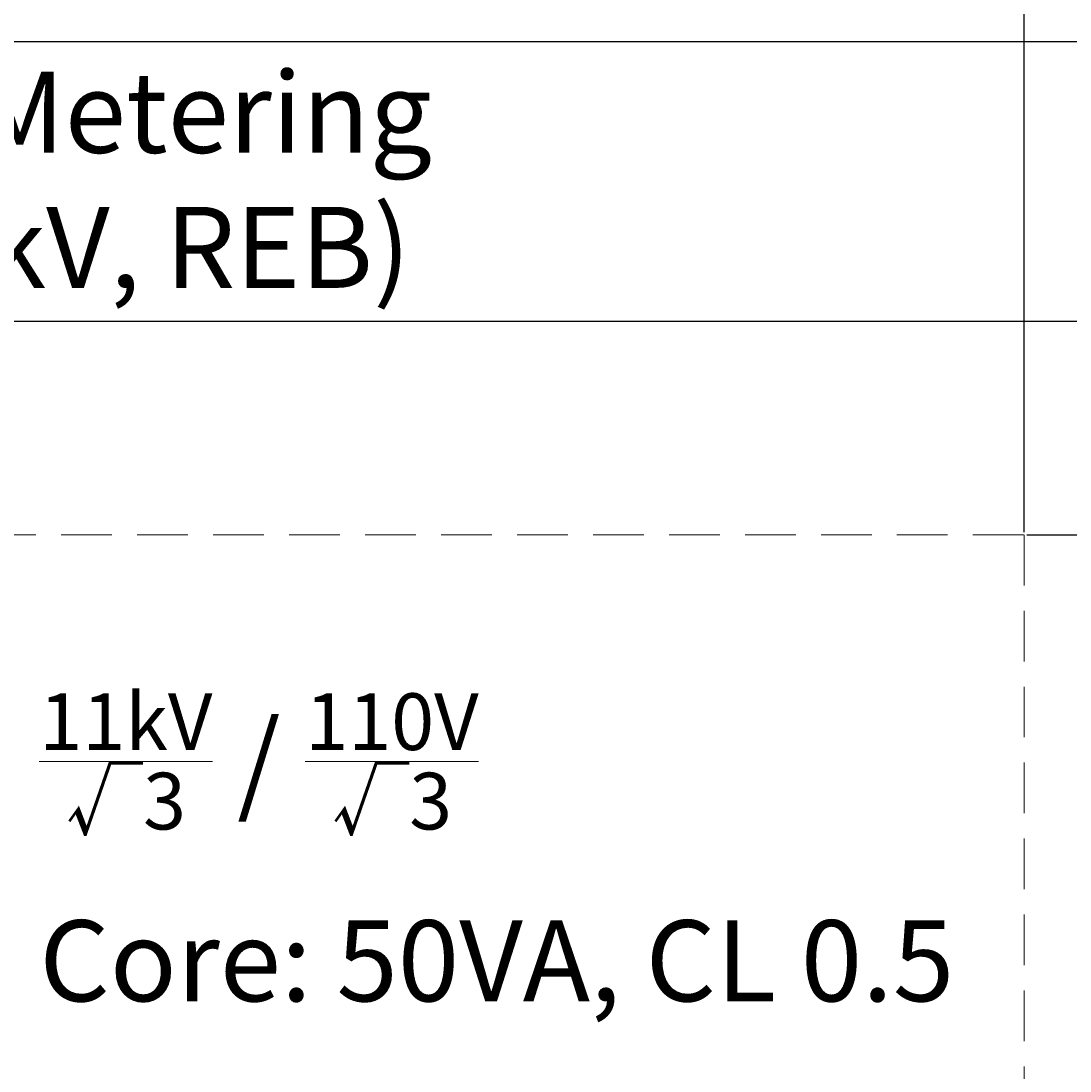
# Model space of a CAD drawing. Units: inches. Extents: x 412 to 584, y 208 to 437.
# Tile 26 of 28: x 514 to 540, y 387 to 413. Entities that reach past the tile are written whole.
import ezdxf

# ---------------------------------------------------------------- set-up
doc = ezdxf.new("R2010")
doc.units = ezdxf.units.IN
doc.header["$MEASUREMENT"] = 0
doc.linetypes.add('HIDDEN', pattern=[0.375, 0.25, -0.125])
for name, color, linetype, lineweight in [('A-ANNO-DIMS', 2, 'Continuous', 18), ('E-ANNO-TEXT', 7, 'Continuous', 18), ('E-ENCL-HIDN', 3, 'HIDDEN', 18)]:
    doc.layers.add(name, color=color, linetype=linetype, lineweight=lineweight)
doc.styles.get("Standard").update_dxf_attribs({"font": 'arial.ttf'})
doc.dimstyles.get("Standard").update_dxf_attribs({"dimtxt": 0.18, "dimasz": 0.18, "dimexe": 0.18, "dimexo": 0.0625, "dimgap": 0.09, "dimtad": 0, "dimtih": 1, "dimtoh": 1, "dimdec": 4, "dimzin": 0, "dimdsep": 46, "dimtxsty": 'Standard', "dimcen": 0.09, "dimadec": 0, "dimazin": 0, "dimtfac": 1, "dimtdec": 4, "dimtofl": 0, "dimtmove": 0, "dimatfit": 3, "dimfxl": 1, "dimtolj": 1, "dimtzin": 0, "dimarcsym": 0})

# ---------------------------------------------------------------- blocks, each defined once
blk = doc.blocks.new('*D17')
at = {"layer": 'A-ANNO-DIMS', "color": 0, "lineweight": -2, "transparency": 16777216}
for p, q in [((497.715, 426.185), (583.674, 426.185)), ((583.494, 426.005), (583.494, 323.031)), ((583.494, 219.693), (583.494, 322.667)), ((550.198, 219.513), (583.674, 219.513))]:
    blk.add_line(p, q, dxfattribs=at)
at = {"layer": 'A-ANNO-DIMS', "color": 0, "transparency": 16777216}
for points in [[(583.464, 426.005), (583.524, 426.005), (583.494, 426.185)], [(583.464, 219.693), (583.524, 219.693), (583.494, 219.513)]]:
    blk.add_solid(points, dxfattribs=at)
at = {"layer": 'Defpoints', "color": 0, "transparency": 16777216}
for p in [(497.652, 426.185), (550.135, 219.513), (583.494, 219.513)]:
    blk.add_point(p, dxfattribs=at)
at = {"layer": 'A-ANNO-DIMS', "color": 0, "transparency": 16777216, "insert": (583.494, 322.849), "char_height": 0.18, "attachment_point": 5}
blk.add_mtext('\\A1;206.67', dxfattribs=at)
blk = doc.blocks.new('*D20')
at = {"layer": 'A-ANNO-DIMS', "color": 0, "lineweight": -2, "transparency": 16777216}
for p, q in [((507.316, 412.35), (583.674, 412.35)), ((583.494, 412.17), (583.494, 406.444)), ((583.494, 400.355), (583.494, 406.08)), ((538.681, 400.175), (583.674, 400.175))]:
    blk.add_line(p, q, dxfattribs=at)
at = {"layer": 'A-ANNO-DIMS', "color": 0, "transparency": 16777216}
for points in [[(583.464, 412.17), (583.524, 412.17), (583.494, 412.35)], [(583.464, 400.355), (583.524, 400.355), (583.494, 400.175)]]:
    blk.add_solid(points, dxfattribs=at)
at = {"layer": 'Defpoints', "color": 0, "transparency": 16777216}
for p in [(507.254, 412.35), (538.619, 400.175), (583.494, 400.175)]:
    blk.add_point(p, dxfattribs=at)
at = {"layer": 'A-ANNO-DIMS', "color": 0, "transparency": 16777216, "insert": (583.494, 406.262), "char_height": 0.18, "attachment_point": 5}
blk.add_mtext('\\A1;12.175', dxfattribs=at)
blk = doc.blocks.new('*D21')
at = {"layer": 'A-ANNO-DIMS', "color": 0, "lineweight": -2, "transparency": 16777216}
for p, q in [((466.104, 400.237), (466.104, 437.465)), ((538.619, 400.237), (538.619, 437.465)), ((466.284, 437.285), (501.986, 437.285)), ((538.439, 437.285), (502.737, 437.285))]:
    blk.add_line(p, q, dxfattribs=at)
at = {"layer": 'A-ANNO-DIMS', "color": 0, "transparency": 16777216}
for points in [[(466.284, 437.315), (466.284, 437.255), (466.104, 437.285)], [(538.439, 437.315), (538.439, 437.255), (538.619, 437.285)]]:
    blk.add_solid(points, dxfattribs=at)
at = {"layer": 'Defpoints', "color": 0, "transparency": 16777216}
for p in [(538.619, 437.285), (466.104, 400.175), (538.619, 400.175)]:
    blk.add_point(p, dxfattribs=at)
at = {"layer": 'A-ANNO-DIMS', "color": 0, "transparency": 16777216, "insert": (502.361, 437.285), "char_height": 0.18, "attachment_point": 5}
blk.add_mtext('\\A1;72.51', dxfattribs=at)
blk = doc.blocks.new('*D28')
at = {"layer": 'A-ANNO-DIMS', "color": 0, "lineweight": -2, "transparency": 16777216}
for p, q in [((450.562, 256.635), (450.562, 437.465)), ((555.796, 256.635), (555.796, 437.465)), ((450.742, 437.285), (502.724, 437.285)), ((555.616, 437.285), (503.634, 437.285))]:
    blk.add_line(p, q, dxfattribs=at)
at = {"layer": 'A-ANNO-DIMS', "color": 0, "transparency": 16777216}
for points in [[(450.742, 437.315), (450.742, 437.255), (450.562, 437.285)], [(555.616, 437.315), (555.616, 437.255), (555.796, 437.285)]]:
    blk.add_solid(points, dxfattribs=at)
at = {"layer": 'Defpoints', "color": 0, "transparency": 16777216}
for p in [(555.796, 437.285), (450.562, 256.573), (555.796, 256.573)]:
    blk.add_point(p, dxfattribs=at)
at = {"layer": 'A-ANNO-DIMS', "color": 0, "transparency": 16777216, "insert": (503.179, 437.285), "char_height": 0.18, "attachment_point": 5}
blk.add_mtext('\\A1;105.23', dxfattribs=at)
blk = doc.blocks.new('*D32')
at = {"layer": 'A-ANNO-DIMS', "color": 0, "lineweight": -2, "transparency": 16777216}
for p, q in [((507.316, 412.35), (583.674, 412.35)), ((583.494, 412.17), (583.494, 409.081)), ((583.494, 405.628), (583.494, 408.717)), ((507.316, 405.448), (583.674, 405.448))]:
    blk.add_line(p, q, dxfattribs=at)
at = {"layer": 'A-ANNO-DIMS', "color": 0, "transparency": 16777216}
for points in [[(583.464, 412.17), (583.524, 412.17), (583.494, 412.35)], [(583.464, 405.628), (583.524, 405.628), (583.494, 405.448)]]:
    blk.add_solid(points, dxfattribs=at)
at = {"layer": 'Defpoints', "color": 0, "transparency": 16777216}
for p in [(507.254, 412.35), (507.254, 405.448), (583.494, 405.448)]:
    blk.add_point(p, dxfattribs=at)
at = {"layer": 'A-ANNO-DIMS', "color": 0, "transparency": 16777216, "insert": (583.494, 408.899), "char_height": 0.18, "attachment_point": 5}
blk.add_mtext('\\A1;6.902', dxfattribs=at)

msp = doc.modelspace()

# ---------------------------------------------------------------- linework, layer by layer
at = {"layer": 'E-ENCL-HIDN', "ltscale": 5}
msp.add_lwpolyline([(466.1037, 400.175), (538.6186, 400.175), (538.6186, 360.1961), (466.1037, 360.1961)], close=True, dxfattribs=at)

# ---------------------------------------------------------------- texts
at = {"layer": 'E-ANNO-TEXT', "char_height": 2, "attachment_point": 1}
for s, width, heights, insert in [('\\pxqc;HT Metering\\P(11kV, REB)', 20.444042, [7.5463], (506.0251, 411.601)), ('\\A1;{\\H0.7x;\\S11kV/√3;\\fMS Shell Dlg 2|b0|i0|c0|p0;\\H1.42857x; / \\fArial|b0|i0|c0|p34;\\H0.7x;\\S110V/√3;}\\PCore: 50VA, CL 0.5', 30.155276, [10.2349], (514.3116, 396.2607))]:
    msp.add_mtext_dynamic_manual_height_columns(s, width=width, gutter_width=1, heights=heights, dxfattribs=dict(at, insert=insert))

# ---------------------------------------------------------------- dimensions: what is measured, and where the dimension line sits
at = {"layer": 'A-ANNO-DIMS'}
for base, p1, p2, picture, middle in [((555.7959, 437.2847), (450.562, 256.5729), (555.7959, 256.5729), '*D28', (503.1789, 437.2847)), ((538.6186, 437.2847), (466.1037, 400.175), (538.6186, 400.175), '*D21', (502.3612, 437.2847))]:
    dim = msp.add_linear_dim(base=base, p1=p1, p2=p2, dimstyle='Standard', override={"dimdec": 2, "dimlfac": 1, "dimrnd": 0, "dimzin": 0, "dimdsep": 46, "dimlunit": 2}, dxfattribs=at)
    dim.commit()
    dim.dimension.update_dxf_attribs({"geometry": picture, "text_midpoint": middle})
for base, p1, p2, override, picture, middle in [((583.4937, 219.5133), (497.6523, 426.1847), (550.1351, 219.5133), {"dimdec": 2, "dimlfac": 1, "dimrnd": 0, "dimzin": 0, "dimdsep": 46, "dimlunit": 2}, '*D17', (583.4937, 322.849)), ((583.4937, 400.175), (507.2538, 412.3496), (538.6186, 400.175), {"dimdec": 3, "dimlfac": 1, "dimrnd": 0, "dimzin": 0, "dimdsep": 46, "dimlunit": 2}, '*D20', (583.4937, 406.2623)), ((583.4937, 405.448), (507.2538, 412.3496), (507.2538, 405.448), {"dimdec": 3, "dimlfac": 1, "dimrnd": 0, "dimzin": 0, "dimdsep": 46, "dimlunit": 2}, '*D32', (583.4937, 408.8988))]:
    dim = msp.add_linear_dim(base=base, p1=p1, p2=p2, angle=90, dimstyle='Standard', override=override, dxfattribs=at)
    dim.commit()
    dim.dimension.update_dxf_attribs({"geometry": picture, "text_midpoint": middle})

doc.saveas('drawing.dxf')
